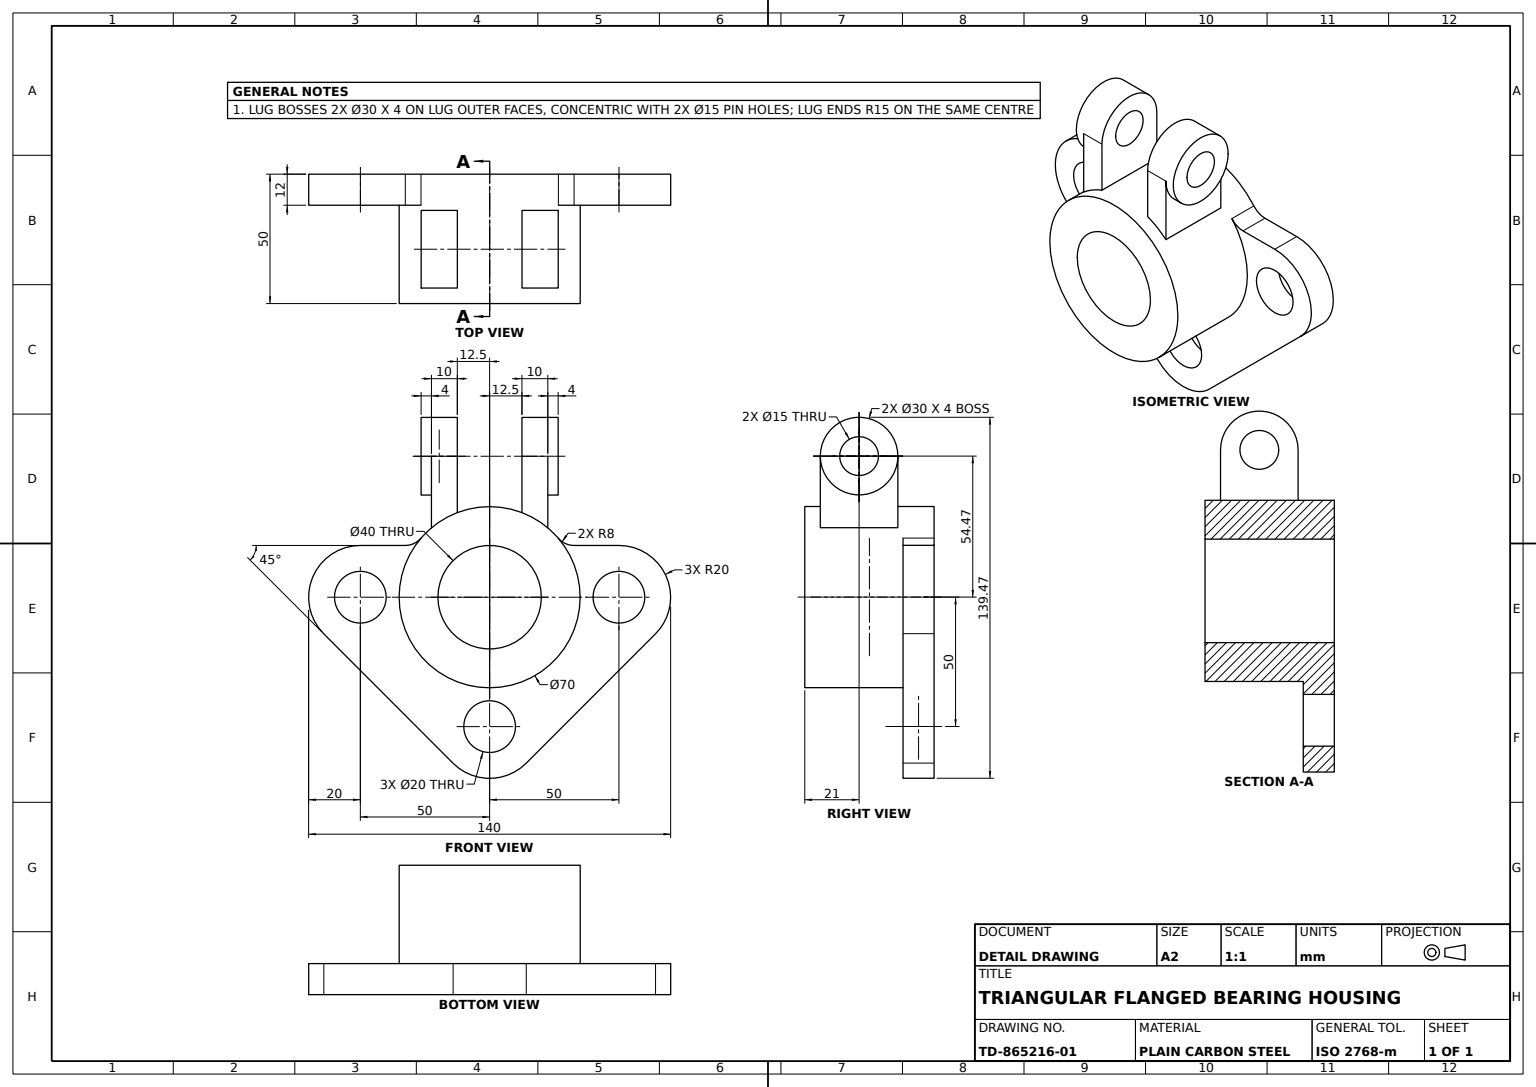
from build123d import *
from build123d.topology import SkipClean

# Parameters (mm, degrees)
HUB_SKETCH_R                   = 35
BEARING_HUB_DEPTH              = 50
BORE_SKETCH_R                  = 20
BEARING_BORE_40_DEPTH          = 71.356236397
MOUNTING_FLANGE_DEPTH          = 12
FLANGE_FILLETS_R8_R            = 8
FLANGE_HOLES_SKETCH_R          = 10
FLANGE_MOUNTING_HOLES_20_DEPTH = 12
CLEVIS_LUG_1_DEPTH             = 10
LUG_1_BOSS_SKETCH_R            = 15
LUG_1_BOSS_30_DEPTH            = 4
CLEVIS_START                   = -10
CLEVIS_LUG_2_DEPTH             = 10
LUG_START                      = 4
LUG_2_BOSS_SKETCH_R            = 15
LUG_2_BOSS_30_DEPTH            = 4
PIN_HOLE_SKETCH_R              = 7.5
LUG_PIN_HOLE_15_DEPTH          = 130.275867818


with BuildPart() as part:
    # Hub Sketch → Bearing Hub (new body)
    with BuildSketch(Plane.XY):
        Circle(HUB_SKETCH_R)
    extrude(amount=-BEARING_HUB_DEPTH)

    # Bore Sketch → Bearing Bore Ø40 (cut, through all)
    with BuildSketch(Plane.XY):
        Circle(BORE_SKETCH_R)
    extrude(amount=-BEARING_BORE_40_DEPTH, mode=Mode.SUBTRACT)

    # Flange Profile Sketch → Mounting Flange (add)
    with BuildSketch(Plane.XY.offset(-38)):
        with BuildLine():
            Line((-50, 20), (-28.722813233, 20))
            ThreePointArc((-28.722813233, 20), (0, -35), (28.722813233, 20))
            Line((28.722813233, 20), (50, 20))
            ThreePointArc((50, 20), (68.47759065, 7.653668647), (64.142135624, -14.142135624))
            Line((64.142135624, -14.142135624), (14.142135624, -64.142135624))
            ThreePointArc((14.142135624, -64.142135624), (0, -70), (-14.142135624, -64.142135624))
            Line((-14.142135624, -64.142135624), (-64.142135624, -14.142135624))
            ThreePointArc((-64.142135624, -14.142135624), (-68.47759065, 7.653668647), (-50, 20))
        make_face()
    extrude(amount=-MOUNTING_FLANGE_DEPTH)

    # Flange Fillets R8
    flange_fillets_r8_edges = [part.edges().sort_by_distance(p)[0] for p in [
        (-28.722813233, 20, -44),
        (28.722813233, 20, -44),
    ]]
    fillet(flange_fillets_r8_edges, radius=FLANGE_FILLETS_R8_R)

    # Flange Holes Sketch → Flange Mounting Holes Ø20 (cut)
    with BuildSketch(Plane.XY.offset(-38)):
        with Locations((50, 0)):
            Circle(FLANGE_HOLES_SKETCH_R)
        with Locations((0, -50)):
            Circle(FLANGE_HOLES_SKETCH_R)
        with Locations((-50, 0)):
            Circle(FLANGE_HOLES_SKETCH_R)
    extrude(amount=-FLANGE_MOUNTING_HOLES_20_DEPTH, mode=Mode.SUBTRACT)

    # Lug 1 Profile Sketch → Clevis Lug 1 (add)
    with BuildSketch(Plane(origin=(12.5, 0, 0), x_dir=(0, 0, -1), z_dir=(1, 0, 0))):
        with BuildLine():
            Line((6, 54.471410374), (6, 26.471410374))
            Line((6, 26.471410374), (36, 26.471410374))
            Line((36, 26.471410374), (36, 54.471410374))
            ThreePointArc((36, 54.471410374), (21, 69.471410374), (6, 54.471410374))
        make_face()
    extrude(amount=CLEVIS_LUG_1_DEPTH)

    # Lug 1 Boss Sketch → Lug 1 Boss Ø30 (add)
    with BuildSketch(Plane(origin=(22.5, 0, 0), x_dir=(0, 0, -1), z_dir=(1, 0, 0))):
        with Locations((21, 54.471410374)):
            Circle(LUG_1_BOSS_SKETCH_R)
    extrude(amount=LUG_1_BOSS_30_DEPTH)

    # Lug 2 Profile Sketch → Clevis Lug 2 (add)
    with BuildSketch(Plane(origin=(-12.5, 0, 0), x_dir=(0, 0, -1), z_dir=(1, 0, 0)).offset(CLEVIS_START)):
        with BuildLine():
            Line((36, 54.471410374), (36, 26.471410374))
            Line((36, 26.471410374), (6, 26.471410374))
            Line((6, 26.471410374), (6, 54.471410374))
            ThreePointArc((6, 54.471410374), (21, 69.471410374), (36, 54.471410374))
        make_face()
    extrude(amount=CLEVIS_LUG_2_DEPTH)

    # Lug 2 Boss Sketch → Lug 2 Boss Ø30 (add)
    with SkipClean():  # the faces are left unmerged after this step: merging them gives an invalid solid
        with BuildSketch(Plane.ZY.offset(22.5).offset(LUG_START)):
            with Locations(Location((-21, 54.471410374, 0), (0, 0, 180))):
                Circle(LUG_2_BOSS_SKETCH_R)
        extrude(amount=-LUG_2_BOSS_30_DEPTH)

    # Pin Hole Sketch → Lug Pin Hole Ø15 (cut, through all)
    with SkipClean():  # the faces are left unmerged after this step: merging them gives an invalid solid
        with BuildSketch(Plane(origin=(26.5, 0, 0), x_dir=(0, 0, -1), z_dir=(1, 0, 0))):
            with Locations((21, 54.471410374)):
                Circle(PIN_HOLE_SKETCH_R)
        extrude(amount=-LUG_PIN_HOLE_15_DEPTH, mode=Mode.SUBTRACT)


solid = part.part
